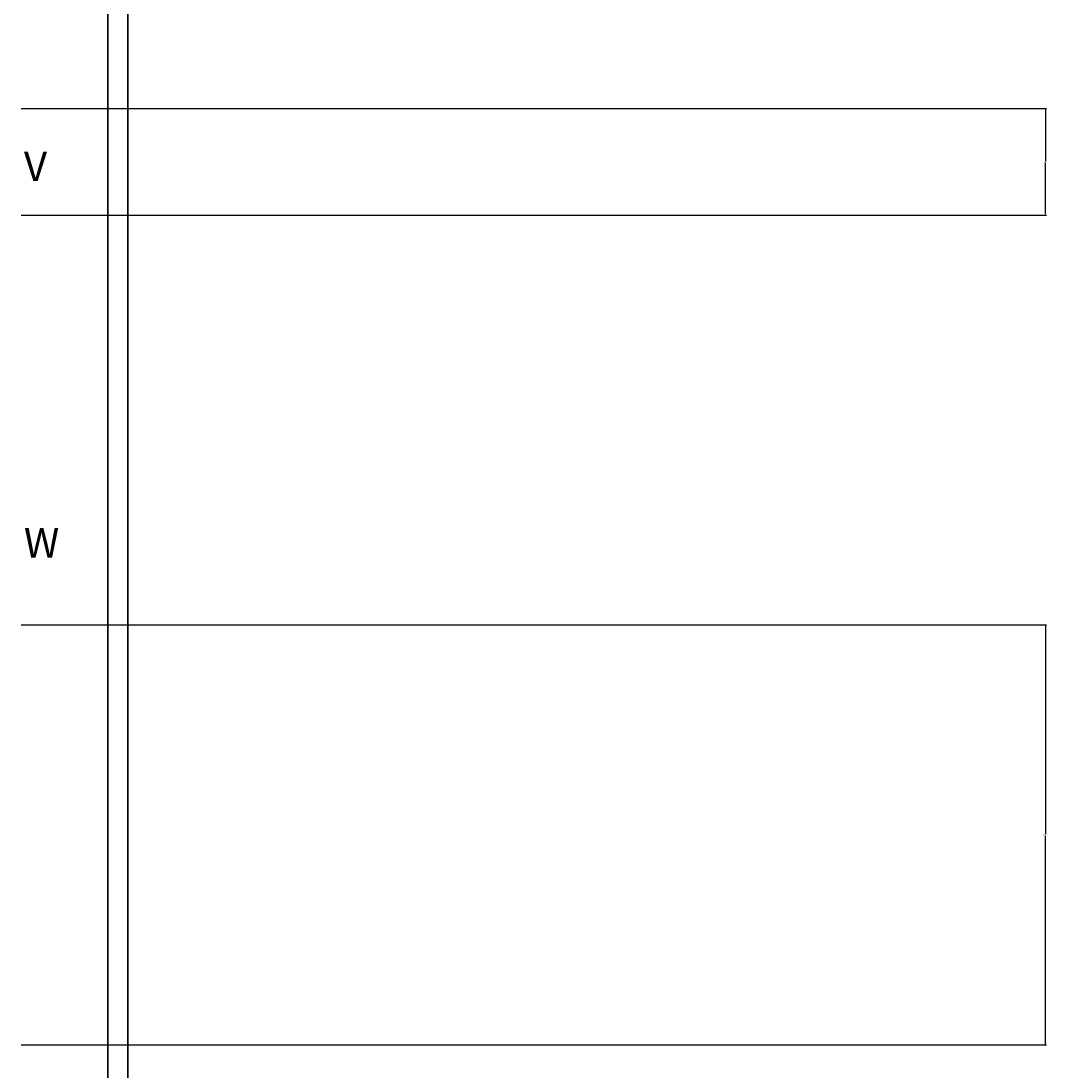
# Model space of a CAD drawing. Units: inches. Extents: x 338 to 1188, y -996 to 127.
# Tile 13 of 15: x 957 to 1188, y -622 to -385. Entities that reach past the tile are written whole.
import ezdxf

# ---------------------------------------------------------------- set-up
doc = ezdxf.new("R2010")
doc.units = ezdxf.units.IN
doc.header["$MEASUREMENT"] = 0
for name, color, linetype, lineweight in [('A-ANNO-DIMS', 5, 'Continuous', 18), ('A-ANNO-TEXT', 7, 'Continuous', 18), ('C-PROP', 1, 'Continuous', 35)]:
    doc.layers.add(name, color=color, linetype=linetype, lineweight=lineweight)
doc.styles.get("Standard").update_dxf_attribs({"font": 'arial.ttf'})
doc.dimstyles.get("Standard").update_dxf_attribs({"dimtxt": 0.18, "dimasz": 0.18, "dimexe": 0.18, "dimexo": 0.0625, "dimgap": 0.09, "dimtad": 0, "dimtih": 1, "dimtoh": 1, "dimdec": 1, "dimzin": 0, "dimdsep": 46, "dimlunit": 4, "dimtxsty": 'Standard', "dimcen": 0.09, "dimadec": 0, "dimazin": 0, "dimtfac": 1, "dimtdec": 1, "dimtofl": 0, "dimtmove": 0, "dimatfit": 3, "dimfxl": 1, "dimtolj": 1, "dimtzin": 0, "dimarcsym": 0})

# ---------------------------------------------------------------- blocks, each defined once
blk = doc.blocks.new('*D41')
at = {"layer": 'A-ANNO-DIMS', "color": 0, "lineweight": -2, "transparency": 16777216}
for p, q in [((957.03, -405.07), (1187.6, -405.07)), ((1187.42, -405.25), (1187.42, -416.89)), ((1187.42, -428.89), (1187.42, -417.26)), ((957.03, -429.07), (1187.6, -429.07))]:
    blk.add_line(p, q, dxfattribs=at)
at = {"layer": 'A-ANNO-DIMS', "color": 0, "transparency": 16777216}
for points in [[(1187.39, -405.25), (1187.45, -405.25), (1187.42, -405.07)], [(1187.39, -428.89), (1187.45, -428.89), (1187.42, -429.07)]]:
    blk.add_solid(points, dxfattribs=at)
at = {"layer": 'Defpoints', "color": 0, "transparency": 16777216}
for p in [(956.96, -405.07), (956.96, -429.07), (1187.42, -429.07)]:
    blk.add_point(p, dxfattribs=at)
at = {"layer": 'A-ANNO-DIMS', "color": 0, "transparency": 16777216, "insert": (1187.42, -417.07), "char_height": 0.18, "attachment_point": 5}
blk.add_mtext('\\A1;2\'-0"', dxfattribs=at)
blk = doc.blocks.new('*D47')
at = {"layer": 'A-ANNO-DIMS', "color": 0, "lineweight": -2, "transparency": 16777216}
for p, q in [((759.67, -755.17), (759.67, 67.25)), ((759.85, 67.07), (867.68, 67.07)), ((976.28, 67.07), (868.46, 67.07)), ((976.46, -755.17), (976.46, 67.25))]:
    blk.add_line(p, q, dxfattribs=at)
at = {"layer": 'A-ANNO-DIMS', "color": 0, "transparency": 16777216}
for points in [[(759.85, 67.1), (759.85, 67.04), (759.67, 67.07)], [(976.28, 67.1), (976.28, 67.04), (976.46, 67.07)]]:
    blk.add_solid(points, dxfattribs=at)
at = {"layer": 'Defpoints', "color": 0, "transparency": 16777216}
for p in [(976.46, 67.07), (759.67, -755.23), (976.46, -755.23)]:
    blk.add_point(p, dxfattribs=at)
at = {"layer": 'A-ANNO-DIMS', "color": 0, "transparency": 16777216, "insert": (868.07, 67.07), "char_height": 0.18, "attachment_point": 5}
blk.add_mtext('\\A1;18\'-1"', dxfattribs=at)
blk = doc.blocks.new('*D52')
at = {"layer": 'A-ANNO-DIMS', "color": 0, "lineweight": -2, "transparency": 16777216}
for p, q in [((957.03, -521.22), (1187.6, -521.22)), ((1187.42, -521.4), (1187.42, -568.29)), ((1187.42, -615.55), (1187.42, -568.66)), ((957.03, -615.73), (1187.6, -615.73))]:
    blk.add_line(p, q, dxfattribs=at)
at = {"layer": 'A-ANNO-DIMS', "color": 0, "transparency": 16777216}
for points in [[(1187.39, -521.4), (1187.45, -521.4), (1187.42, -521.22)], [(1187.39, -615.55), (1187.45, -615.55), (1187.42, -615.73)]]:
    blk.add_solid(points, dxfattribs=at)
at = {"layer": 'Defpoints', "color": 0, "transparency": 16777216}
for p in [(956.96, -521.22), (956.96, -615.73), (1187.42, -615.73)]:
    blk.add_point(p, dxfattribs=at)
at = {"layer": 'A-ANNO-DIMS', "color": 0, "transparency": 16777216, "insert": (1187.42, -568.48), "char_height": 0.18, "attachment_point": 5}
blk.add_mtext('\\A1;7\'-10 1/2"', dxfattribs=at)

msp = doc.modelspace()

# ---------------------------------------------------------------- linework, layer by layer
at = {"layer": 'C-PROP'}
for p, q in [((980.96, 8.27), (980.96, -807.73)), ((976.46, 3.77), (976.46, -803.23))]:
    msp.add_line(p, q, dxfattribs=at)

# ---------------------------------------------------------------- texts
at = {"layer": 'A-ANNO-TEXT'}
for s, p in [('V', (957.61, -421.43)), ('W', (957.61, -506.1))]:
    msp.add_text(s, height=6.65, dxfattribs=at).set_placement(p)

# ---------------------------------------------------------------- dimensions: what is measured, and where the dimension line sits
at = {"layer": 'A-ANNO-DIMS'}
dim = msp.add_linear_dim(base=(976.46, 67.07), p1=(759.67, -755.23), p2=(976.46, -755.23), dimstyle='Standard', override={"dimdec": 1, "dimlfac": 1, "dimrnd": 0, "dimzin": 1, "dimdsep": 46, "dimlunit": 4, "dimfrac": 2}, dxfattribs=at)
dim.commit()
dim.dimension.update_dxf_attribs({"geometry": '*D47', "text_midpoint": (868.07, 67.07)})
for base, p1, p2, picture, middle in [((1187.42, -429.07), (956.96, -405.07), (956.96, -429.07), '*D41', (1187.42, -417.07)), ((1187.42, -615.73), (956.96, -521.22), (956.96, -615.73), '*D52', (1187.42, -568.48))]:
    dim = msp.add_linear_dim(base=base, p1=p1, p2=p2, angle=90, dimstyle='Standard', override={"dimdec": 1, "dimlfac": 1, "dimrnd": 0, "dimzin": 1, "dimdsep": 46, "dimlunit": 4, "dimfrac": 2}, dxfattribs=at)
    dim.commit()
    dim.dimension.update_dxf_attribs({"geometry": picture, "text_midpoint": middle})

doc.saveas('drawing.dxf')
